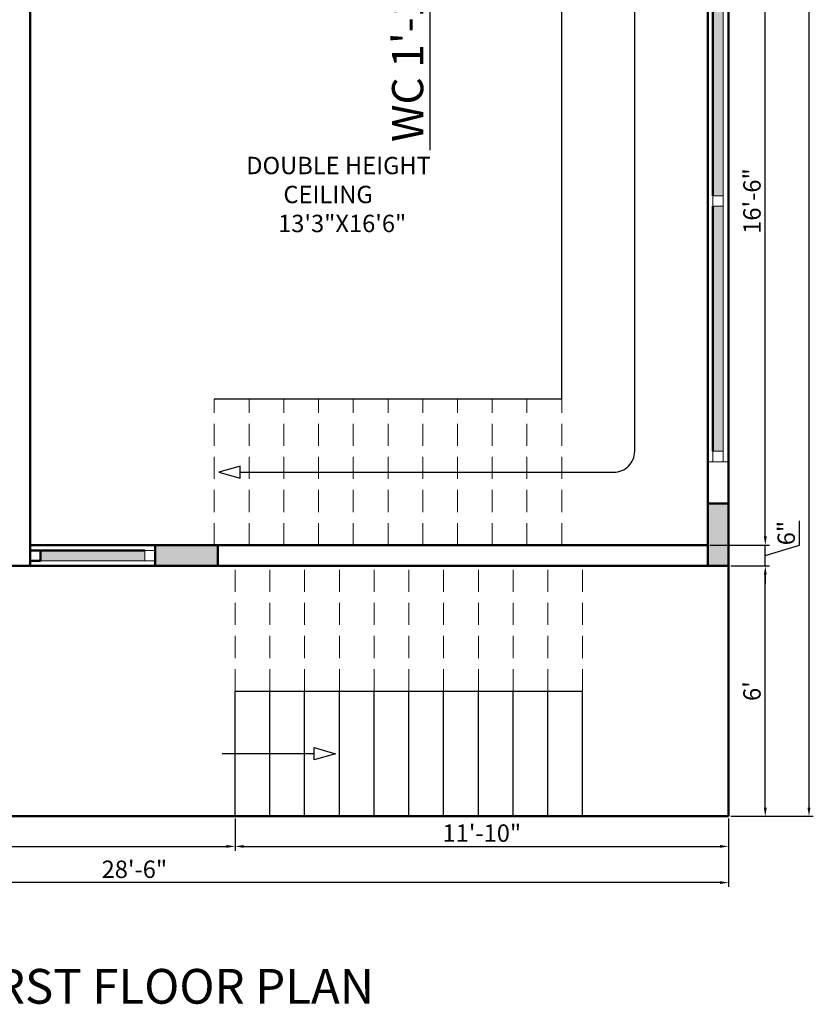
# Model space of a CAD drawing. Units: inches. Extents: x 3064 to 19385, y 846 to 15425.
# Tile 42 of 108: x 5329 to 5557, y 846 to 1129. Entities that reach past the tile are written whole.
import ezdxf

# ---------------------------------------------------------------- set-up
doc = ezdxf.new("R2010")
doc.units = ezdxf.units.IN
doc.linetypes.add('DASHED', pattern=[19.05, 12.7, -6.35])
for name, color, linetype, lineweight in [('A-ANNO-DIMS', 2, 'Continuous', 18), ('A-ANNO-TEXT', 7, 'Continuous', 25), ('A-AREA-IDEN', 3, 'Continuous', 18), ('A-COLS', 1, 'Continuous', 35), ('A-FLOR-STRS', 2, 'Continuous', 25), ('A-FLOR-STRS-OVHD', 2, 'DASHED', 18), ('A-GLAZ', 4, 'Continuous', 18), ('A-WALL', 7, 'Continuous', 50)]:
    doc.layers.add(name, color=color, linetype=linetype, lineweight=lineweight)
doc.styles.get("Standard").update_dxf_attribs({"font": 'arial.ttf'})
doc.dimstyles.new('ISO-25', dxfattribs={"dimtxt": 9, "dimasz": 2.5, "dimexe": 1.25, "dimexo": 0.625, "dimtad": 1, "dimdec": 1, "dimlunit": 3, "dimtxsty": 'Standard', "dimcen": 2.5, "dimadec": 0, "dimazin": 0, "dimtfac": 1, "dimtdec": 1, "dimtmove": 0, "dimatfit": 3, "dimfxl": 1, "dimarcsym": 0})

# ---------------------------------------------------------------- blocks, each defined once
blk = doc.blocks.new('*D77')
at = {"layer": 'A-ANNO-DIMS', "color": 0, "lineweight": -2, "transparency": 16777216}
for p, q in [((5191.02, 899.47), (5191.02, 890.17)), ((5391.02, 899.47), (5391.02, 890.17)), ((5193.52, 891.42), (5388.52, 891.42))]:
    blk.add_line(p, q, dxfattribs=at)
at = {"layer": 'A-ANNO-DIMS', "color": 0, "transparency": 16777216}
for points in [[(5193.52, 891.84), (5193.52, 891.01), (5191.02, 891.42)], [(5388.52, 891.84), (5388.52, 891.01), (5391.02, 891.42)]]:
    blk.add_solid(points, dxfattribs=at)
at = {"layer": 'Defpoints', "color": 0, "transparency": 16777216}
for p in [(5191.02, 900.1), (5391.02, 900.1), (5391.02, 891.42)]:
    blk.add_point(p, dxfattribs=at)
at = {"layer": 'A-ANNO-DIMS', "color": 0, "transparency": 16777216, "insert": (5291.02, 894.6), "char_height": 5, "attachment_point": 5}
blk.add_mtext('16\'-8"', dxfattribs=at)
blk = doc.blocks.new('*D78')
at = {"layer": 'A-ANNO-DIMS', "color": 0, "lineweight": -2, "transparency": 16777216}
for p, q in [((5391.02, 899.47), (5391.02, 890.17)), ((5533.02, 899.47), (5533.02, 890.17)), ((5393.52, 891.42), (5530.52, 891.42))]:
    blk.add_line(p, q, dxfattribs=at)
at = {"layer": 'A-ANNO-DIMS', "color": 0, "transparency": 16777216}
for points in [[(5393.52, 891.84), (5393.52, 891.01), (5391.02, 891.42)], [(5530.52, 891.84), (5530.52, 891.01), (5533.02, 891.42)]]:
    blk.add_solid(points, dxfattribs=at)
at = {"layer": 'Defpoints', "color": 0, "transparency": 16777216}
for p in [(5391.02, 900.1), (5533.02, 900.1), (5533.02, 891.42)]:
    blk.add_point(p, dxfattribs=at)
at = {"layer": 'A-ANNO-DIMS', "color": 0, "transparency": 16777216, "insert": (5462.02, 894.6), "char_height": 5, "attachment_point": 5}
blk.add_mtext('11\'-10"', dxfattribs=at)
blk = doc.blocks.new('*D79')
at = {"layer": 'A-ANNO-DIMS', "color": 0, "lineweight": -2, "transparency": 16777216}
for p, q in [((5191.02, 899.47), (5191.02, 879.76)), ((5533.02, 899.47), (5533.02, 879.76)), ((5530.52, 881.01), (5193.52, 881.01))]:
    blk.add_line(p, q, dxfattribs=at)
at = {"layer": 'A-ANNO-DIMS', "color": 0, "transparency": 16777216}
for points in [[(5193.52, 881.43), (5193.52, 880.6), (5191.02, 881.01)], [(5530.52, 881.43), (5530.52, 880.6), (5533.02, 881.01)]]:
    blk.add_solid(points, dxfattribs=at)
at = {"layer": 'Defpoints', "color": 0, "transparency": 16777216}
for p in [(5191.02, 900.1), (5533.02, 900.1), (5191.02, 881.01)]:
    blk.add_point(p, dxfattribs=at)
at = {"layer": 'A-ANNO-DIMS', "color": 0, "transparency": 16777216, "insert": (5362.02, 884.19), "char_height": 5, "attachment_point": 5}
blk.add_mtext('28\'-6"', dxfattribs=at)
blk = doc.blocks.new('*D80')
at = {"layer": 'A-ANNO-DIMS', "color": 0, "lineweight": -2, "transparency": 16777216}
for p, q in [((5533.64, 972.1), (5544.85, 972.1)), ((5543.6, 902.6), (5543.6, 969.6)), ((5533.64, 900.1), (5544.85, 900.1))]:
    blk.add_line(p, q, dxfattribs=at)
at = {"layer": 'A-ANNO-DIMS', "color": 0, "transparency": 16777216}
for points in [[(5543.18, 969.6), (5544.02, 969.6), (5543.6, 972.1)], [(5543.18, 902.6), (5544.02, 902.6), (5543.6, 900.1)]]:
    blk.add_solid(points, dxfattribs=at)
at = {"layer": 'Defpoints', "color": 0, "transparency": 16777216}
for p in [(5533.02, 972.1), (5543.6, 972.1), (5533.02, 900.1)]:
    blk.add_point(p, dxfattribs=at)
at = {"layer": 'A-ANNO-DIMS', "color": 0, "transparency": 16777216, "insert": (5540.42, 936.1), "char_height": 5, "attachment_point": 5, "rotation": 90}
blk.add_mtext("6'", dxfattribs=at)
blk = doc.blocks.new('*D81')
at = {"layer": 'A-ANNO-DIMS', "color": 0, "lineweight": -2, "transparency": 16777216}
for p, q in [((5543.6, 980.6), (5543.6, 983.1)), ((5553.45, 978.05), (5553.45, 985.07)), ((5527.64, 978.1), (5544.85, 978.1)), ((5543.6, 972.1), (5543.6, 978.1)), ((5543.6, 972.1), (5543.6, 978.1)), ((5543.6, 975.1), (5553.45, 978.05)), ((5533.64, 972.1), (5544.85, 972.1)), ((5543.6, 969.6), (5543.6, 967.1))]:
    blk.add_line(p, q, dxfattribs=at)
at = {"layer": 'A-ANNO-DIMS', "color": 0, "transparency": 16777216}
for points in [[(5543.18, 980.6), (5544.02, 980.6), (5543.6, 978.1)], [(5543.18, 969.6), (5544.02, 969.6), (5543.6, 972.1)]]:
    blk.add_solid(points, dxfattribs=at)
at = {"layer": 'Defpoints', "color": 0, "transparency": 16777216}
for p in [(5527.02, 978.1), (5543.6, 978.1), (5533.02, 972.1)]:
    blk.add_point(p, dxfattribs=at)
at = {"layer": 'A-ANNO-DIMS', "color": 0, "transparency": 16777216, "insert": (5550.27, 981.56), "char_height": 5, "attachment_point": 5, "rotation": 90}
blk.add_mtext('6"', dxfattribs=at)
blk = doc.blocks.new('*D82')
at = {"layer": 'A-ANNO-DIMS', "color": 0, "lineweight": -2, "transparency": 16777216}
for p, q in [((5533.64, 1176.1), (5544.85, 1176.1)), ((5543.6, 980.6), (5543.6, 1173.6)), ((5527.64, 978.1), (5544.85, 978.1))]:
    blk.add_line(p, q, dxfattribs=at)
at = {"layer": 'A-ANNO-DIMS', "color": 0, "transparency": 16777216}
for points in [[(5543.18, 1173.6), (5544.02, 1173.6), (5543.6, 1176.1)], [(5543.18, 980.6), (5544.02, 980.6), (5543.6, 978.1)]]:
    blk.add_solid(points, dxfattribs=at)
at = {"layer": 'Defpoints', "color": 0, "transparency": 16777216}
for p in [(5533.02, 1176.1), (5543.6, 1176.1), (5527.02, 978.1)]:
    blk.add_point(p, dxfattribs=at)
at = {"layer": 'A-ANNO-DIMS', "color": 0, "transparency": 16777216, "insert": (5540.42, 1077.1), "char_height": 5, "attachment_point": 5, "rotation": 90}
blk.add_mtext('16\'-6"', dxfattribs=at)
blk = doc.blocks.new('*D88')
at = {"layer": 'A-ANNO-DIMS', "color": 0, "lineweight": -2, "transparency": 16777216}
for p, q in [((5533.64, 1392.1), (5557.42, 1392.1)), ((5556.17, 1389.6), (5556.17, 902.6)), ((5533.64, 900.1), (5557.42, 900.1))]:
    blk.add_line(p, q, dxfattribs=at)
at = {"layer": 'A-ANNO-DIMS', "color": 0, "transparency": 16777216}
for points in [[(5555.75, 1389.6), (5556.59, 1389.6), (5556.17, 1392.1)], [(5555.75, 902.6), (5556.59, 902.6), (5556.17, 900.1)]]:
    blk.add_solid(points, dxfattribs=at)
at = {"layer": 'Defpoints', "color": 0, "transparency": 16777216}
for p in [(5533.02, 1392.1), (5533.02, 900.1), (5556.17, 900.1)]:
    blk.add_point(p, dxfattribs=at)
at = {"layer": 'A-ANNO-DIMS', "color": 0, "transparency": 16777216, "insert": (5553.04, 1146.1), "char_height": 5, "attachment_point": 5, "rotation": 90}
blk.add_mtext("41'", dxfattribs=at)
blk = doc.blocks.new('WIN-1800-PAIR')
h = blk.add_hatch(color=256)
h.dxf.hatch_style = 1
h.paths.add_polyline_path([(0, 0), (3, 0), (3, 70.5), (0, 70.5)])
h.paths.add_polyline_path([(3, 144), (0, 144), (0, 73.5), (3, 73.5)])
blk.add_line((3, 144), (3, 73.5))
blk.add_lwpolyline([(3, 144), (0, 144), (0, 147), (3, 147)], close=True)
blk = doc.blocks.new('WIN-900')
blk.add_line((0, 0), (30, 0))
blk.add_lwpolyline([(30, 0), (30, 3), (33, 3), (33, 0)], close=True)
blk = doc.blocks.new('WIN-2000')
blk.add_line((3, 0), (3, 70.5))
blk.add_lwpolyline([(3, 70.5), (0, 70.5), (0, 73.5), (3, 73.5)], close=True)
blk = doc.blocks.new('*D405')
at = {"layer": 'A-ANNO-DIMS', "color": 0, "lineweight": -2, "transparency": 16777216}
for p, q in [((5449.79, 1204.19), (5445.85, 1204.19)), ((5447.1, 1201.69), (5447.1, 1184.6)), ((5449.79, 1182.1), (5445.85, 1182.1)), ((5447.1, 1182.1), (5447.1, 1091.69))]:
    blk.add_line(p, q, dxfattribs=at)
at = {"layer": 'A-ANNO-DIMS', "color": 0, "transparency": 16777216}
for points in [[(5446.69, 1201.69), (5447.52, 1201.69), (5447.1, 1204.19)], [(5446.69, 1184.6), (5447.52, 1184.6), (5447.1, 1182.1)]]:
    blk.add_solid(points, dxfattribs=at)
at = {"layer": 'Defpoints', "color": 0, "transparency": 16777216}
for p in [(5450.42, 1204.19), (5447.1, 1182.1), (5450.42, 1182.1)]:
    blk.add_point(p, dxfattribs=at)
at = {"layer": 'A-ANNO-DIMS', "color": 0, "transparency": 16777216, "insert": (5441.83, 1135.64), "char_height": 9, "attachment_point": 5, "rotation": 90}
blk.add_mtext('WC 1\'-10" TYP.', dxfattribs=at)

msp = doc.modelspace()

# ---------------------------------------------------------------- hatches: boundary and pattern name
at = {"layer": 'A-COLS'}
h = msp.add_hatch(color=256, dxfattribs=at)
h.dxf.hatch_style = 1
h.paths.add_polyline_path([(5533.02, 972.1), (5533.02, 990.1), (5527.02, 990.1), (5527.02, 972.1)])
h = msp.add_hatch(color=256, dxfattribs=at)
h.dxf.hatch_style = 1
h.paths.add_polyline_path([(5386.02, 978.1), (5368.02, 978.1), (5368.02, 972.1), (5386.02, 972.1)])
at = {"layer": 'A-GLAZ'}
h = msp.add_hatch(color=256, dxfattribs=at)
h.dxf.hatch_style = 1
h.paths.add_polyline_path([(5335.02, 976.6), (5335.02, 973.6), (5365.02, 973.6), (5365.02, 976.6)])

# ---------------------------------------------------------------- linework, layer by layer
at = {"layer": 'A-FLOR-STRS'}
for p, q in [((5485.02, 1020.1), (5485.02, 1176.1)), ((5485.02, 1020.1), (5385.02, 1020.1)), ((5391.02, 900.1), (5391.02, 936.1)), ((5391.02, 936.1), (5491.02, 936.1)), ((5401.02, 900.1), (5401.02, 936.1)), ((5411.02, 900.1), (5411.02, 936.1)), ((5421.02, 900.1), (5421.02, 936.1)), ((5431.02, 900.1), (5431.02, 936.1)), ((5441.02, 900.1), (5441.02, 936.1)), ((5451.02, 900.1), (5451.02, 936.1)), ((5461.02, 900.1), (5461.02, 936.1)), ((5471.02, 900.1), (5471.02, 936.1)), ((5481.02, 900.1), (5481.02, 936.1)), ((5491.02, 900.1), (5491.02, 936.1)), ((5413.72, 918.1), (5387.33, 918.1))]:
    msp.add_line(p, q, dxfattribs=at)
msp.add_lwpolyline([(5392.51, 999.1), (5500.02, 999.1, 0.414214), (5506.02, 1005.1), (5506.02, 1149.1, 0.414214), (5500.02, 1155.1), (5373.02, 1155.1)], format="xyb", dxfattribs=at)
for points in [[(5386.31, 999.1), (5392.51, 997.36), (5392.51, 1000.83)], [(5419.91, 918.1), (5413.72, 916.36), (5413.72, 919.83)]]:
    msp.add_lwpolyline(points, close=True, dxfattribs=at)
at = {"layer": 'A-FLOR-STRS-OVHD', "ltscale": 0.5}
for p, q in [((5385.02, 978.1), (5385.02, 1020.1)), ((5395.02, 978.1), (5395.02, 1020.1)), ((5405.02, 978.1), (5405.02, 1020.1)), ((5415.02, 978.1), (5415.02, 1020.1)), ((5425.02, 978.1), (5425.02, 1020.1)), ((5435.02, 978.1), (5435.02, 1020.1)), ((5445.02, 978.1), (5445.02, 1020.1)), ((5455.02, 978.1), (5455.02, 1020.1)), ((5465.02, 978.1), (5465.02, 1020.1)), ((5475.02, 978.1), (5475.02, 1020.1)), ((5485.02, 978.1), (5485.02, 1020.1)), ((5391.02, 936.1), (5391.02, 972.1)), ((5401.02, 936.1), (5401.02, 972.1)), ((5411.02, 936.1), (5411.02, 972.1)), ((5421.02, 936.1), (5421.02, 972.1)), ((5431.02, 936.1), (5431.02, 972.1)), ((5441.02, 936.1), (5441.02, 972.1)), ((5451.02, 936.1), (5451.02, 972.1)), ((5461.02, 936.1), (5461.02, 972.1)), ((5471.02, 936.1), (5471.02, 972.1)), ((5481.02, 936.1), (5481.02, 972.1)), ((5491.02, 936.1), (5491.02, 972.1))]:
    msp.add_line(p, q, dxfattribs=at)
at = {"layer": 'A-GLAZ'}
msp.add_line((5533.02, 1002.1), (5527.02, 1002.1), dxfattribs=at)
msp.add_line((5533.02, 1002.1), (5527.02, 1002.1), dxfattribs=at)
msp.add_lwpolyline([(5531.52, 1002.1), (5528.52, 1002.1), (5528.52, 1005.1), (5531.52, 1005.1)], close=True, dxfattribs=at)
at = {"layer": 'A-WALL'}
for p, q in [((5533.02, 900.1), (5533.02, 1392.1)), ((5527.02, 978.1), (5527.02, 1176.1)), ((5528.52, 1149.1), (5528.52, 1078.6)), ((5332.02, 1140.1), (5332.02, 972.1)), ((5528.52, 1005.1), (5528.52, 1075.6)), ((5527.02, 978.1), (5332.02, 978.1)), ((5332.02, 972.1), (5332.02, 978.1)), ((5368.02, 972.1), (5368.02, 978.1)), ((5368.02, 972.1), (5368.02, 978.1)), ((5335.02, 976.6), (5365.02, 976.6)), ((5533.02, 972.1), (5191.02, 972.1)), ((5191.02, 900.1), (5533.02, 900.1))]:
    msp.add_line(p, q, dxfattribs=at)
for points in [[(5533.02, 972.1), (5533.02, 990.1), (5527.02, 990.1), (5527.02, 972.1)], [(5386.02, 978.1), (5368.02, 978.1), (5368.02, 972.1), (5386.02, 972.1)], [(5332.02, 973.6), (5332.02, 976.6), (5335.02, 976.6), (5335.02, 973.6)]]:
    msp.add_lwpolyline(points, close=True, dxfattribs=at)

# ---------------------------------------------------------------- block references
at = {"layer": 'A-GLAZ'}
for name, p in [('WIN-1800-PAIR', (5528.52, 1005.1)), ('WIN-2000', (5528.52, 1005.1)), ('WIN-900', (5335.02, 973.6))]:
    msp.add_blockref(name, p, dxfattribs=at)

# ---------------------------------------------------------------- texts
at = {"layer": 'A-ANNO-TEXT', "insert": (5310.36, 856.17), "char_height": 10, "attachment_point": 1}
msp.add_mtext_dynamic_manual_height_columns('FIRST FLOOR PLAN', width=200.9739, gutter_width=12.5, heights=[0], dxfattribs=at)
at = {"layer": 'A-AREA-IDEN', "insert": (5394.22, 1089.82), "char_height": 5, "attachment_point": 1}
msp.add_mtext_dynamic_manual_height_columns('DOUBLE HEIGHT \\P       CEILING            \\P      13\'3"X16\'6"', width=57.0817, gutter_width=12.5, heights=[0], dxfattribs=at)

# ---------------------------------------------------------------- dimensions: what is measured, and where the dimension line sits
at = {"layer": 'A-ANNO-DIMS'}
for base, p1, p2, override, picture, middle in [((5556.17, 900.1), (5533.02, 1392.1), (5533.02, 900.1), {"dimtxt": 5, "dimclrd": 0, "dimclre": 0, "dimclrt": 0}, '*D88', (5553.04, 1146.1)), ((5543.6, 1176.1), (5527.02, 978.1), (5533.02, 1176.1), {"dimtxt": 5, "dimclrd": 0, "dimclre": 0, "dimclrt": 0, "dimtmove": 1}, '*D82', (5540.42, 1077.1)), ((5543.6, 978.1), (5533.02, 972.1), (5527.02, 978.1), {"dimtxt": 5, "dimclrd": 0, "dimclre": 0, "dimclrt": 0, "dimtmove": 1}, '*D81', (5550.27, 978.68)), ((5543.6, 972.1), (5533.02, 900.1), (5533.02, 972.1), {"dimtxt": 5, "dimclrd": 0, "dimclre": 0, "dimclrt": 0}, '*D80', (5540.42, 936.1))]:
    dim = msp.add_linear_dim(base=base, p1=p1, p2=p2, angle=90, dimstyle='ISO-25', override=override, dxfattribs=at)
    dim.commit()
    dim.dimension.update_dxf_attribs({"geometry": picture, "text_midpoint": middle})
dim = msp.add_linear_dim(base=(5447.1, 1182.1), p1=(5450.42, 1204.19), p2=(5450.42, 1182.1), angle=270, text='WC <> TYP.', dimstyle='ISO-25', override={"dimdec": 1, "dimrnd": 0, "dimzin": 1, "dimlunit": 4, "dimfrac": 2}, dxfattribs=at)
dim.commit()
dim.dimension.update_dxf_attribs({"geometry": '*D405', "text_midpoint": (5441.83, 1135.64)})
for base, p1, p2, override, picture, middle in [((5391.02, 891.42), (5191.02, 900.1), (5391.02, 900.1), {"dimtxt": 5, "dimclrd": 0, "dimclre": 0, "dimclrt": 0}, '*D77', (5291.02, 894.6)), ((5191.02, 881.01), (5533.02, 900.1), (5191.02, 900.1), {"dimtxt": 5, "dimclrd": 0, "dimclre": 0, "dimclrt": 0}, '*D79', (5362.02, 884.19)), ((5533.02, 891.42), (5391.02, 900.1), (5533.02, 900.1), {"dimtxt": 5, "dimclrd": 0, "dimclre": 0, "dimclrt": 0, "dimtmove": 1}, '*D78', (5462.02, 894.6))]:
    dim = msp.add_linear_dim(base=base, p1=p1, p2=p2, dimstyle='ISO-25', override=override, dxfattribs=at)
    dim.commit()
    dim.dimension.update_dxf_attribs({"geometry": picture, "text_midpoint": middle})

doc.saveas('drawing.dxf')
